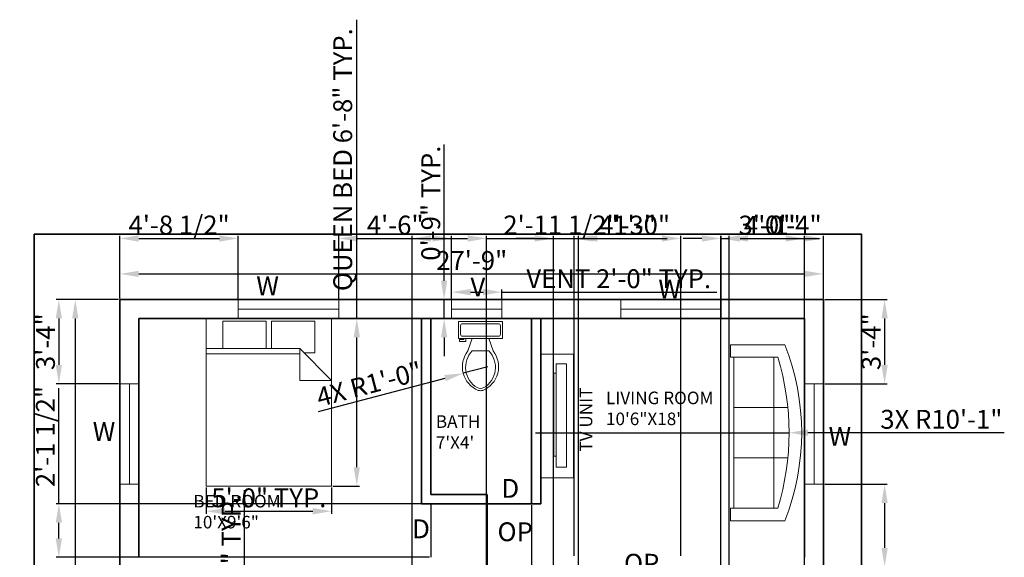
# Model space of a CAD drawing. Units: inches. Extents: x 53076 to 53578, y 41072 to 41816.
# Tile 4 of 4: x 53099 to 53569, y 41560 to 41816. Entities that reach past the tile are written whole.
import ezdxf

# ---------------------------------------------------------------- set-up
doc = ezdxf.new("R2010")
doc.units = ezdxf.units.IN
for name, color, linetype, lineweight in [('A-ANNO-DIMS', 2, 'Continuous', 18), ('A-ANNO-TEXT', 7, 'Continuous', 18), ('A-ANNO-TTLB', 7, 'Continuous', 35), ('A-AREA-IDEN', 7, 'Continuous', 18), ('A-DOOR', 3, 'Continuous', 25), ('A-EQPM', 8, 'Continuous', 18), ('A-FLOR-CASE', 9, 'Continuous', 18), ('A-FLOR-FIXT', 9, 'Continuous', 18), ('A-FURN', 8, 'Continuous', 18), ('A-GLAZ', 4, 'Continuous', 18), ('A-WALL', 7, 'Continuous', 35)]:
    doc.layers.add(name, color=color, linetype=linetype, lineweight=lineweight)
doc.styles.get("Standard").update_dxf_attribs({"font": 'arial.ttf'})
doc.dimstyles.new('ISO-25', dxfattribs={"dimtxt": 9, "dimasz": 9, "dimexe": 1.25, "dimexo": 0.625, "dimtad": 1, "dimdec": 1, "dimrnd": 9, "dimlunit": 3, "dimtxsty": 'Standard', "dimcen": 2.5, "dimadec": 0, "dimazin": 0, "dimtfac": 1, "dimtdec": 1, "dimtmove": 0, "dimatfit": 3, "dimfxl": 1, "dimarcsym": 0})

# ---------------------------------------------------------------- blocks, each defined once
blk = doc.blocks.new('*D1')
at = {"layer": 'A-ANNO-DIMS', "color": 0, "lineweight": -2, "transparency": 16777216}
for p, q in [((53146.81, 41683.28), (53146.81, 41696.2)), ((53482.81, 41683.28), (53482.81, 41696.2)), ((53155.81, 41694.95), (53473.81, 41694.95))]:
    blk.add_line(p, q, dxfattribs=at)
at = {"layer": 'A-ANNO-DIMS', "color": 0, "transparency": 16777216}
for points in [[(53155.81, 41696.45), (53155.81, 41693.45), (53146.81, 41694.95)], [(53473.81, 41696.45), (53473.81, 41693.45), (53482.81, 41694.95)]]:
    blk.add_solid(points, dxfattribs=at)
at = {"layer": 'Defpoints', "color": 0, "transparency": 16777216}
for p in [(53482.81, 41694.95), (53146.81, 41682.66), (53482.81, 41682.66)]:
    blk.add_point(p, dxfattribs=at)
at = {"layer": 'A-ANNO-DIMS', "color": 0, "transparency": 16777216, "insert": (53314.81, 41700.17), "char_height": 9, "attachment_point": 5}
blk.add_mtext('27\'-9"', dxfattribs=at)
blk = doc.blocks.new('*D2')
at = {"layer": 'A-ANNO-DIMS', "color": 0, "lineweight": -2, "transparency": 16777216}
for p, q in [((53146.18, 41682.66), (53124.21, 41682.66)), ((53125.46, 41673.66), (53125.46, 41161.66)), ((53146.18, 41152.66), (53124.21, 41152.66))]:
    blk.add_line(p, q, dxfattribs=at)
at = {"layer": 'A-ANNO-DIMS', "color": 0, "transparency": 16777216}
for points in [[(53123.96, 41673.66), (53126.96, 41673.66), (53125.46, 41682.66)], [(53123.96, 41161.66), (53126.96, 41161.66), (53125.46, 41152.66)]]:
    blk.add_solid(points, dxfattribs=at)
at = {"layer": 'Defpoints', "color": 0, "transparency": 16777216}
for p in [(53146.81, 41682.66), (53125.46, 41152.66), (53146.81, 41152.66)]:
    blk.add_point(p, dxfattribs=at)
at = {"layer": 'A-ANNO-DIMS', "color": 0, "transparency": 16777216, "insert": (53120.23, 41417.66), "char_height": 9, "attachment_point": 5, "rotation": 90}
blk.add_mtext('44\'-3"', dxfattribs=at)
blk = doc.blocks.new('Bed - Queen')
for p, q in [((0, -80.00003), (0, 0)), ((0, 0), (59.99999, 0)), ((59.99999, 0), (59.99999, -80.00003)), ((7.99999, -1.2), (28.79998, -1.2)), ((7.99999, -14.4), (7.99999, -1.2)), ((28.79998, -1.2), (28.79998, -14.4)), ((31.19999, -1.2), (51.99999, -1.2)), ((31.19999, -14.4), (31.19999, -1.2)), ((51.99999, -1.2), (51.99999, -16.4)), ((0, -14.4), (44.8, -14.4)), ((44.8, -16.8), (0, -16.8)), ((59.99999, -29.6), (44.8, -14.4)), ((44.8, -14.4), (44.8, -29.6)), ((51.99999, -16.4), (46.79936, -16.4)), ((44.8, -29.6), (59.99999, -29.6)), ((59.99999, -80.00003), (0, -80.00003))]:
    blk.add_line(p, q)
blk = doc.blocks.new('Sofa - Roundback 7 ft.')
for p, q in [((-12.00002, -32.4421), (-12.00003, -6.5971)), ((11.99997, -32.4421), (11.99998, -6.5971)), ((-36.000027, -34), (-36.000027, -11.4696)), ((-35.999844, -13.3819), (35.9998, -13.3819)), ((35.99998, -34), (35.99998, -11.4696)), ((-36.000027, -32.4421), (35.99998, -32.4421))]:
    blk.add_line(p, q)
for points in [[(-36.000027, -34), (-42.000027, -34), (-42.000027, -8)], [(41.99998, -8), (41.99998, -34), (35.99998, -34)]]:
    blk.add_lwpolyline(points)
for centre, radius, start, end in [((0, -114.25), 114.25, 68.43141, 111.5686), ((-0.00001, -127.1968), 121.1968, 72.72033, 107.2797)]:
    blk.add_arc(centre, radius, start, end)
blk = doc.blocks.new('Toilet - top')
for p, q in [((9.5, -6), (9.5, -2)), ((-10, -8.5), (-8, -8.5)), ((-10, -9.5), (-10, -8.5)), ((-8, -8.5), (-8, -8)), ((-7, -8), (-7, -9.5)), ((-4, -8), (-6, -14)), ((4, -8), (6, -14)), ((-7, -9.5), (-10, -9.5)), ((4, -14), (-4, -14))]:
    blk.add_line(p, q)
blk.add_lwpolyline([(10.5, -8), (10.5, 0), (-10.5, 0), (-10.5, -8)], close=True)
for points in [[(-9.5, -2), (-9.5, -6)], [(8.5, -1), (-8.5, -1)], [(-8.5, -7), (8.5, -7)]]:
    blk.add_lwpolyline(points)
for centre, radius, start, end in [((-8.62, -1.88), 0.884, 81.8699, 188.1301), ((8.62, -1.88), 0.884, 351.8699, 98.1301), ((-8.62, -6.12), 0.884, 171.8699, 278.1301), ((8.62, -6.12), 0.884, 261.8699, 8.1301), ((3.52, -21.58), 12.17, 141.4691, 247.9714), ((4.2, -21.82), 11.33, 136.3677, 238.9468), ((-3.52, -21.58), 12.17, 292.0284, 38.5307), ((-4.2, -21.82), 11.33, 301.053, 43.6321), ((0, -27.88), 4, 245.7318, 294.2682), ((0, -29), 4, 254.8605, 285.1395)]:
    blk.add_arc(centre, radius, start, end)
blk = doc.blocks.new('WIN-48IN')
for p, q in [((0, 48), (9, 48)), ((4.5, 48), (4.5, 0)), ((0, 0), (9, 0))]:
    blk.add_line(p, q)
blk = doc.blocks.new('VENT-24IN')
for p, q in [((0, 9), (0, 0)), ((24, 9), (24, 0)), ((0, 4.5), (24, 4.5))]:
    blk.add_line(p, q)
blk = doc.blocks.new('*D18')
at = {"layer": 'A-ANNO-DIMS', "color": 0, "lineweight": -2, "transparency": 16777216}
for p, q in [((53206.33, 41493.74), (53206.33, 41591.64)), ((53207.95, 41484.74), (53205.08, 41484.74)), ((53206.33, 41469.74), (53206.33, 41484.74)), ((53207.95, 41469.74), (53205.08, 41469.74)), ((53206.33, 41460.74), (53206.33, 41451.74))]:
    blk.add_line(p, q, dxfattribs=at)
at = {"layer": 'A-ANNO-DIMS', "color": 0, "transparency": 16777216}
for points in [[(53204.83, 41493.74), (53207.83, 41493.74), (53206.33, 41484.74)], [(53204.83, 41460.74), (53207.83, 41460.74), (53206.33, 41469.74)]]:
    blk.add_solid(points, dxfattribs=at)
at = {"layer": 'Defpoints', "color": 0, "transparency": 16777216}
for p in [(53206.33, 41484.74), (53208.58, 41484.74), (53208.58, 41469.74)]:
    blk.add_point(p, dxfattribs=at)
at = {"layer": 'A-ANNO-DIMS', "color": 0, "transparency": 16777216, "insert": (53201.05, 41547.19), "char_height": 9, "attachment_point": 5, "rotation": 90}
blk.add_mtext('SINK 1\'-3" TYP.', dxfattribs=at)
blk = doc.blocks.new('*D24')
at = {"layer": 'A-ANNO-DIMS', "color": 0, "lineweight": -2, "transparency": 16777216}
for p, q in [((53305.23, 41683.28), (53305.23, 41687.51)), ((53314.23, 41686.26), (53320.23, 41686.26)), ((53329.23, 41683.28), (53329.23, 41687.51)), ((53329.23, 41686.26), (53431.83, 41686.26))]:
    blk.add_line(p, q, dxfattribs=at)
at = {"layer": 'A-ANNO-DIMS', "color": 0, "transparency": 16777216}
for points in [[(53314.23, 41687.76), (53314.23, 41684.76), (53305.23, 41686.26)], [(53320.23, 41687.76), (53320.23, 41684.76), (53329.23, 41686.26)]]:
    blk.add_solid(points, dxfattribs=at)
at = {"layer": 'Defpoints', "color": 0, "transparency": 16777216}
for p in [(53329.23, 41686.26), (53305.23, 41682.66), (53329.23, 41682.66)]:
    blk.add_point(p, dxfattribs=at)
at = {"layer": 'A-ANNO-DIMS', "color": 0, "transparency": 16777216, "insert": (53385.03, 41691.48), "char_height": 9, "attachment_point": 5}
blk.add_mtext('VENT 2\'-0" TYP.', dxfattribs=at)
blk = doc.blocks.new('*D25')
at = {"layer": 'A-ANNO-DIMS', "color": 0, "lineweight": -2, "transparency": 16777216}
for p, q in [((53301.63, 41691.66), (53301.63, 41756.77)), ((53304.61, 41682.66), (53300.38, 41682.66)), ((53301.63, 41673.66), (53301.63, 41682.66)), ((53304.61, 41673.66), (53300.38, 41673.66)), ((53301.63, 41664.66), (53301.63, 41655.66))]:
    blk.add_line(p, q, dxfattribs=at)
at = {"layer": 'A-ANNO-DIMS', "color": 0, "transparency": 16777216}
for points in [[(53300.13, 41691.66), (53303.13, 41691.66), (53301.63, 41682.66)], [(53300.13, 41664.66), (53303.13, 41664.66), (53301.63, 41673.66)]]:
    blk.add_solid(points, dxfattribs=at)
at = {"layer": 'Defpoints', "color": 0, "transparency": 16777216}
for p in [(53301.63, 41682.66), (53305.23, 41682.66), (53305.23, 41673.66)]:
    blk.add_point(p, dxfattribs=at)
at = {"layer": 'A-ANNO-DIMS', "color": 0, "transparency": 16777216, "insert": (53296.41, 41728.71), "char_height": 9, "attachment_point": 5, "rotation": 90}
blk.add_mtext('0\'-9" TYP.', dxfattribs=at)
blk = doc.blocks.new('*D26')
at = {"layer": 'A-ANNO-DIMS', "color": 0, "lineweight": -2, "transparency": 16777216}
for p, q in [((53259.91, 41673.66), (53259.91, 41816.3)), ((53248.53, 41673.66), (53261.16, 41673.66)), ((53259.91, 41602.66), (53259.91, 41664.66)), ((53248.53, 41593.66), (53261.16, 41593.66))]:
    blk.add_line(p, q, dxfattribs=at)
at = {"layer": 'A-ANNO-DIMS', "color": 0, "transparency": 16777216}
for points in [[(53258.41, 41664.66), (53261.41, 41664.66), (53259.91, 41673.66)], [(53258.41, 41602.66), (53261.41, 41602.66), (53259.91, 41593.66)]]:
    blk.add_solid(points, dxfattribs=at)
at = {"layer": 'Defpoints', "color": 0, "transparency": 16777216}
for p in [(53247.91, 41673.66), (53259.91, 41673.66), (53247.91, 41593.66)]:
    blk.add_point(p, dxfattribs=at)
at = {"layer": 'A-ANNO-DIMS', "color": 0, "transparency": 16777216, "insert": (53254.35, 41749.48), "char_height": 9, "attachment_point": 5, "rotation": 90}
blk.add_mtext('QUEEN BED 6\'-8" TYP.', dxfattribs=at)
blk = doc.blocks.new('*D27')
at = {"layer": 'A-ANNO-DIMS', "color": 0, "lineweight": -2, "transparency": 16777216}
for p, q in [((53187.91, 41593.03), (53187.91, 41580.41)), ((53247.91, 41593.03), (53247.91, 41580.41)), ((53196.91, 41581.66), (53238.91, 41581.66))]:
    blk.add_line(p, q, dxfattribs=at)
at = {"layer": 'A-ANNO-DIMS', "color": 0, "transparency": 16777216}
for points in [[(53196.91, 41583.16), (53196.91, 41580.16), (53187.91, 41581.66)], [(53238.91, 41583.16), (53238.91, 41580.16), (53247.91, 41581.66)]]:
    blk.add_solid(points, dxfattribs=at)
at = {"layer": 'Defpoints', "color": 0, "transparency": 16777216}
for p in [(53187.91, 41593.66), (53247.91, 41593.66), (53247.91, 41581.66)]:
    blk.add_point(p, dxfattribs=at)
at = {"layer": 'A-ANNO-DIMS', "color": 0, "transparency": 16777216, "insert": (53217.91, 41586.88), "char_height": 9, "attachment_point": 5}
blk.add_mtext('5\'-0" TYP.', dxfattribs=at)
blk = doc.blocks.new('*D32')
at = {"layer": 'A-ANNO-DIMS', "color": 0, "lineweight": -2, "transparency": 16777216}
for p, q in [((53483.43, 41594.51), (53513.26, 41594.51)), ((53512.01, 41585.51), (53512.01, 41564.16)), ((53483.43, 41555.16), (53513.26, 41555.16)), ((53512.01, 41555.16), (53512.01, 41500.02))]:
    blk.add_line(p, q, dxfattribs=at)
at = {"layer": 'A-ANNO-DIMS', "color": 0, "transparency": 16777216}
for points in [[(53510.51, 41585.51), (53513.51, 41585.51), (53512.01, 41594.51)], [(53510.51, 41564.16), (53513.51, 41564.16), (53512.01, 41555.16)]]:
    blk.add_solid(points, dxfattribs=at)
at = {"layer": 'Defpoints', "color": 0, "transparency": 16777216}
for p in [(53482.81, 41594.51), (53482.81, 41555.16), (53512.01, 41555.16)]:
    blk.add_point(p, dxfattribs=at)
at = {"layer": 'A-ANNO-DIMS', "color": 0, "transparency": 16777216, "insert": (53506.72, 41523.09), "char_height": 9, "attachment_point": 5, "rotation": 90}
blk.add_mtext('3\'-3 1/2"', dxfattribs=at)
blk = doc.blocks.new('*D39')
at = {"layer": 'A-ANNO-DIMS', "color": 0, "lineweight": -2, "transparency": 16777216}
for p, q in [((53146.81, 41683.28), (53146.81, 41713.11)), ((53155.81, 41711.86), (53194.3, 41711.86)), ((53203.3, 41683.28), (53203.3, 41713.11))]:
    blk.add_line(p, q, dxfattribs=at)
at = {"layer": 'A-ANNO-DIMS', "color": 0, "transparency": 16777216}
for points in [[(53155.81, 41713.36), (53155.81, 41710.36), (53146.81, 41711.86)], [(53194.3, 41713.36), (53194.3, 41710.36), (53203.3, 41711.86)]]:
    blk.add_solid(points, dxfattribs=at)
at = {"layer": 'Defpoints', "color": 0, "transparency": 16777216}
for p in [(53203.3, 41711.86), (53146.81, 41682.66), (53203.3, 41682.66)]:
    blk.add_point(p, dxfattribs=at)
at = {"layer": 'A-ANNO-DIMS', "color": 0, "transparency": 16777216, "insert": (53175.05, 41717.13), "char_height": 9, "attachment_point": 5}
blk.add_mtext('4\'-8 1/2"', dxfattribs=at)
blk = doc.blocks.new('*D40')
at = {"layer": 'A-ANNO-DIMS', "color": 0, "lineweight": -2, "transparency": 16777216}
for p, q in [((53251.3, 41683.28), (53251.3, 41713.11)), ((53260.3, 41711.86), (53296.23, 41711.86)), ((53305.23, 41683.28), (53305.23, 41713.11))]:
    blk.add_line(p, q, dxfattribs=at)
at = {"layer": 'A-ANNO-DIMS', "color": 0, "transparency": 16777216}
for points in [[(53260.3, 41713.36), (53260.3, 41710.36), (53251.3, 41711.86)], [(53296.23, 41713.36), (53296.23, 41710.36), (53305.23, 41711.86)]]:
    blk.add_solid(points, dxfattribs=at)
at = {"layer": 'Defpoints', "color": 0, "transparency": 16777216}
for p in [(53305.23, 41711.86), (53251.3, 41682.66), (53305.23, 41682.66)]:
    blk.add_point(p, dxfattribs=at)
at = {"layer": 'A-ANNO-DIMS', "color": 0, "transparency": 16777216, "insert": (53278.27, 41717.08), "char_height": 9, "attachment_point": 5}
blk.add_mtext('4\'-6"', dxfattribs=at)
blk = doc.blocks.new('*D41')
at = {"layer": 'A-ANNO-DIMS', "color": 0, "lineweight": -2, "transparency": 16777216}
for p, q in [((53433.98, 41683.28), (53433.98, 41713.11)), ((53442.98, 41711.86), (53473.81, 41711.86)), ((53482.81, 41683.28), (53482.81, 41713.11))]:
    blk.add_line(p, q, dxfattribs=at)
at = {"layer": 'A-ANNO-DIMS', "color": 0, "transparency": 16777216}
for points in [[(53442.98, 41713.36), (53442.98, 41710.36), (53433.98, 41711.86)], [(53473.81, 41713.36), (53473.81, 41710.36), (53482.81, 41711.86)]]:
    blk.add_solid(points, dxfattribs=at)
at = {"layer": 'Defpoints', "color": 0, "transparency": 16777216}
for p in [(53482.81, 41711.86), (53433.98, 41682.66), (53482.81, 41682.66)]:
    blk.add_point(p, dxfattribs=at)
at = {"layer": 'A-ANNO-DIMS', "color": 0, "transparency": 16777216, "insert": (53458.4, 41717), "char_height": 9, "attachment_point": 5}
blk.add_mtext('4\'-1"', dxfattribs=at)
blk = doc.blocks.new('*D45')
at = {"layer": 'A-ANNO-DIMS', "color": 0, "lineweight": -2, "transparency": 16777216}
for p, q in [((53146.18, 41682.66), (53116.36, 41682.66)), ((53117.61, 41673.66), (53117.61, 41651.51)), ((53146.18, 41642.51), (53116.36, 41642.51))]:
    blk.add_line(p, q, dxfattribs=at)
at = {"layer": 'A-ANNO-DIMS', "color": 0, "transparency": 16777216}
for points in [[(53116.11, 41673.66), (53119.11, 41673.66), (53117.61, 41682.66)], [(53116.11, 41651.51), (53119.11, 41651.51), (53117.61, 41642.51)]]:
    blk.add_solid(points, dxfattribs=at)
at = {"layer": 'Defpoints', "color": 0, "transparency": 16777216}
for p in [(53146.81, 41682.66), (53117.61, 41642.51), (53146.81, 41642.51)]:
    blk.add_point(p, dxfattribs=at)
at = {"layer": 'A-ANNO-DIMS', "color": 0, "transparency": 16777216, "insert": (53112.38, 41662.58), "char_height": 9, "attachment_point": 5, "rotation": 90}
blk.add_mtext('3\'-4"', dxfattribs=at)
blk = doc.blocks.new('*D48')
at = {"layer": 'A-ANNO-DIMS', "color": 0, "lineweight": -2, "transparency": 16777216}
for p, q in [((53483.43, 41682.66), (53513.26, 41682.66)), ((53512.01, 41673.66), (53512.01, 41651.51)), ((53483.43, 41642.51), (53513.26, 41642.51))]:
    blk.add_line(p, q, dxfattribs=at)
at = {"layer": 'A-ANNO-DIMS', "color": 0, "transparency": 16777216}
for points in [[(53510.51, 41673.66), (53513.51, 41673.66), (53512.01, 41682.66)], [(53510.51, 41651.51), (53513.51, 41651.51), (53512.01, 41642.51)]]:
    blk.add_solid(points, dxfattribs=at)
at = {"layer": 'Defpoints', "color": 0, "transparency": 16777216}
for p in [(53482.81, 41682.66), (53482.81, 41642.51), (53512.01, 41642.51)]:
    blk.add_point(p, dxfattribs=at)
at = {"layer": 'A-ANNO-DIMS', "color": 0, "transparency": 16777216, "insert": (53506.78, 41662.58), "char_height": 9, "attachment_point": 5, "rotation": 90}
blk.add_mtext('3\'-4"', dxfattribs=at)
blk = doc.blocks.new('*D52')
at = {"layer": 'A-ANNO-DIMS', "color": 0, "lineweight": -2, "transparency": 16777216}
for p, q in [((53363.81, 41560.28), (53363.81, 41713.11)), ((53372.81, 41711.86), (53405.67, 41711.86)), ((53414.67, 41560.28), (53414.67, 41713.11))]:
    blk.add_line(p, q, dxfattribs=at)
at = {"layer": 'A-ANNO-DIMS', "color": 0, "transparency": 16777216}
for points in [[(53372.81, 41713.36), (53372.81, 41710.36), (53363.81, 41711.86)], [(53405.67, 41713.36), (53405.67, 41710.36), (53414.67, 41711.86)]]:
    blk.add_solid(points, dxfattribs=at)
at = {"layer": 'Defpoints', "color": 0, "transparency": 16777216}
for p in [(53414.67, 41711.86), (53363.81, 41559.66), (53414.67, 41559.66)]:
    blk.add_point(p, dxfattribs=at)
at = {"layer": 'A-ANNO-DIMS', "color": 0, "transparency": 16777216, "insert": (53389.24, 41717.08), "char_height": 9, "attachment_point": 5}
blk.add_mtext('4\'-3"', dxfattribs=at)
blk = doc.blocks.new('*D55')
at = {"layer": 'A-ANNO-DIMS', "color": 0, "lineweight": -2, "transparency": 16777216}
for p, q in [((53322.2, 41589.03), (53322.2, 41122.21)), ((53343.31, 41584.53), (53343.31, 41122.21)), ((53331.2, 41123.46), (53334.31, 41123.46)), ((53343.31, 41123.46), (53376.63, 41123.46))]:
    blk.add_line(p, q, dxfattribs=at)
at = {"layer": 'A-ANNO-DIMS', "color": 0, "transparency": 16777216}
for points in [[(53331.2, 41124.96), (53331.2, 41121.96), (53322.2, 41123.46)], [(53334.31, 41124.96), (53334.31, 41121.96), (53343.31, 41123.46)]]:
    blk.add_solid(points, dxfattribs=at)
at = {"layer": 'Defpoints', "color": 0, "transparency": 16777216}
for p in [(53322.2, 41589.66), (53343.31, 41585.16), (53343.31, 41123.46)]:
    blk.add_point(p, dxfattribs=at)
at = {"layer": 'A-ANNO-DIMS', "color": 0, "transparency": 16777216, "insert": (53364.47, 41128.68), "char_height": 9, "attachment_point": 5}
blk.add_mtext('1\'-9"', dxfattribs=at)
blk = doc.blocks.new('*D56')
at = {"layer": 'A-ANNO-DIMS', "color": 0, "lineweight": -2, "transparency": 16777216}
for p, q in [((53117.61, 41585.16), (53117.61, 41640.46)), ((53294.68, 41585.16), (53116.36, 41585.16)), ((53117.61, 41568.66), (53117.61, 41576.16)), ((53294.68, 41559.66), (53116.36, 41559.66))]:
    blk.add_line(p, q, dxfattribs=at)
at = {"layer": 'A-ANNO-DIMS', "color": 0, "transparency": 16777216}
for points in [[(53116.11, 41576.16), (53119.11, 41576.16), (53117.61, 41585.16)], [(53116.11, 41568.66), (53119.11, 41568.66), (53117.61, 41559.66)]]:
    blk.add_solid(points, dxfattribs=at)
at = {"layer": 'Defpoints', "color": 0, "transparency": 16777216}
for p in [(53117.61, 41585.16), (53295.31, 41585.16), (53295.31, 41559.66)]:
    blk.add_point(p, dxfattribs=at)
at = {"layer": 'A-ANNO-DIMS', "color": 0, "transparency": 16777216, "insert": (53112.33, 41617.31), "char_height": 9, "attachment_point": 5, "rotation": 90}
blk.add_mtext('2\'-1 1/2"', dxfattribs=at)
blk = doc.blocks.new('*D60')
at = {"layer": 'A-ANNO-DIMS', "color": 0, "lineweight": -2, "transparency": 16777216}
for p, q in [((53286.43, 41391.78), (53286.43, 41713.11)), ((53295.43, 41711.86), (53312.81, 41711.86)), ((53321.81, 41374.01), (53321.81, 41713.11)), ((53321.81, 41711.86), (53384.1, 41711.86))]:
    blk.add_line(p, q, dxfattribs=at)
at = {"layer": 'A-ANNO-DIMS', "color": 0, "transparency": 16777216}
for points in [[(53295.43, 41713.36), (53295.43, 41710.36), (53286.43, 41711.86)], [(53312.81, 41713.36), (53312.81, 41710.36), (53321.81, 41711.86)]]:
    blk.add_solid(points, dxfattribs=at)
at = {"layer": 'Defpoints', "color": 0, "transparency": 16777216}
for p in [(53321.81, 41711.86), (53286.43, 41391.16), (53321.81, 41373.39)]:
    blk.add_point(p, dxfattribs=at)
at = {"layer": 'A-ANNO-DIMS', "color": 0, "transparency": 16777216, "insert": (53357.45, 41717.13), "char_height": 9, "attachment_point": 5}
blk.add_mtext('2\'-11 1/2"', dxfattribs=at)
blk = doc.blocks.new('*D61')
at = {"layer": 'A-ANNO-DIMS', "color": 0, "lineweight": -2, "transparency": 16777216}
for p, q in [((53437.81, 41380.28), (53437.81, 41713.11)), ((53446.81, 41711.86), (53464.81, 41711.86)), ((53473.81, 41380.28), (53473.81, 41713.11))]:
    blk.add_line(p, q, dxfattribs=at)
at = {"layer": 'A-ANNO-DIMS', "color": 0, "transparency": 16777216}
for points in [[(53446.81, 41713.36), (53446.81, 41710.36), (53437.81, 41711.86)], [(53464.81, 41713.36), (53464.81, 41710.36), (53473.81, 41711.86)]]:
    blk.add_solid(points, dxfattribs=at)
at = {"layer": 'Defpoints', "color": 0, "transparency": 16777216}
for p in [(53473.81, 41711.86), (53437.81, 41379.66), (53473.81, 41379.66)]:
    blk.add_point(p, dxfattribs=at)
at = {"layer": 'A-ANNO-DIMS', "color": 0, "transparency": 16777216, "insert": (53455.81, 41717.08), "char_height": 9, "attachment_point": 5}
blk.add_mtext('3\'-0"', dxfattribs=at)
blk = doc.blocks.new('*D62')
at = {"layer": 'A-ANNO-DIMS', "color": 0, "lineweight": -2, "transparency": 16777216}
for p, q in [((53344.81, 41711.86), (53335.81, 41711.86)), ((53353.81, 41448.78), (53353.81, 41713.11)), ((53353.81, 41711.86), (53365.81, 41711.86)), ((53365.81, 41448.78), (53365.81, 41713.11)), ((53374.81, 41711.86), (53408.13, 41711.86))]:
    blk.add_line(p, q, dxfattribs=at)
at = {"layer": 'A-ANNO-DIMS', "color": 0, "transparency": 16777216}
for points in [[(53344.81, 41713.36), (53344.81, 41710.36), (53353.81, 41711.86)], [(53374.81, 41713.36), (53374.81, 41710.36), (53365.81, 41711.86)]]:
    blk.add_solid(points, dxfattribs=at)
at = {"layer": 'Defpoints', "color": 0, "transparency": 16777216}
for p in [(53365.81, 41711.86), (53353.81, 41448.16), (53365.81, 41448.16)]:
    blk.add_point(p, dxfattribs=at)
at = {"layer": 'A-ANNO-DIMS', "color": 0, "transparency": 16777216, "insert": (53395.97, 41717.08), "char_height": 9, "attachment_point": 5}
blk.add_mtext('1\'-0"', dxfattribs=at)
blk = doc.blocks.new('*D67')
at = {"layer": 'A-ANNO-DIMS', "color": 0, "lineweight": -2, "transparency": 16777216}
for p, q in [((53424.78, 41711.86), (53415.78, 41711.86)), ((53433.78, 41514.52), (53433.78, 41713.11)), ((53433.78, 41711.86), (53437.81, 41711.86)), ((53437.81, 41517.49), (53437.81, 41713.11)), ((53446.81, 41711.86), (53480.98, 41711.86))]:
    blk.add_line(p, q, dxfattribs=at)
at = {"layer": 'A-ANNO-DIMS', "color": 0, "transparency": 16777216}
for points in [[(53424.78, 41713.36), (53424.78, 41710.36), (53433.78, 41711.86)], [(53446.81, 41713.36), (53446.81, 41710.36), (53437.81, 41711.86)]]:
    blk.add_solid(points, dxfattribs=at)
at = {"layer": 'Defpoints', "color": 0, "transparency": 16777216}
for p in [(53437.81, 41711.86), (53437.81, 41516.86), (53433.78, 41513.89)]:
    blk.add_point(p, dxfattribs=at)
at = {"layer": 'A-ANNO-DIMS', "color": 0, "transparency": 16777216, "insert": (53468.39, 41717.08), "char_height": 9, "attachment_point": 5}
blk.add_mtext('0\'-4"', dxfattribs=at)
blk = doc.blocks.new('*D71')
at = {"layer": 'A-ANNO-DIMS', "color": 0, "lineweight": -2, "transparency": 16777216}
for p, q in [((53345.22, 41619.13), (53466.41, 41619.13)), ((53569.19, 41619.13), (53475.41, 41619.13))]:
    blk.add_line(p, q, dxfattribs=at)
at = {"layer": 'A-ANNO-DIMS', "color": 0, "transparency": 16777216}
blk.add_solid([(53475.41, 41620.63), (53475.41, 41617.63), (53466.41, 41619.13)], dxfattribs=at)
at = {"layer": 'Defpoints', "color": 0, "transparency": 16777216}
for p in [(53345.22, 41619.13), (53466.41, 41619.13)]:
    blk.add_point(p, dxfattribs=at)
at = {"layer": 'A-ANNO-DIMS', "color": 0, "transparency": 16777216, "insert": (53539.13, 41624.36), "char_height": 9, "attachment_point": 5, "rotation": 0.0001}
blk.add_mtext('3X R10\'-1"', dxfattribs=at)
blk = doc.blocks.new('*D73')
at = {"layer": 'A-ANNO-DIMS', "color": 0, "lineweight": -2, "transparency": 16777216}
for p, q in [((53322.53, 41650.59), (53310.76, 41647.5)), ((53241.62, 41629.33), (53302.05, 41645.21))]:
    blk.add_line(p, q, dxfattribs=at)
at = {"layer": 'A-ANNO-DIMS', "color": 0, "transparency": 16777216}
blk.add_solid([(53301.67, 41646.66), (53302.44, 41643.76), (53310.76, 41647.5)], dxfattribs=at)
at = {"layer": 'Defpoints', "color": 0, "transparency": 16777216}
for p in [(53322.53, 41650.59), (53310.76, 41647.5)]:
    blk.add_point(p, dxfattribs=at)
at = {"layer": 'A-ANNO-DIMS', "color": 0, "transparency": 16777216, "insert": (53266.16, 41641.18), "char_height": 9, "attachment_point": 5, "rotation": 14.7186}
blk.add_mtext('4X R1\'-0"', dxfattribs=at)

msp = doc.modelspace()

# ---------------------------------------------------------------- linework, layer by layer
at = {"layer": 'A-ANNO-TTLB'}
msp.add_lwpolyline([(53105.85, 41713.9), (53500.98, 41713.9), (53500.98, 41125.46), (53105.85, 41125.46)], close=True, dxfattribs=at)
at = {"layer": 'A-DOOR'}
msp.add_line((53295.31, 41585.16), (53295.31, 41559.66), dxfattribs=at)
at = {"layer": 'A-EQPM'}
for p, q in [((53355.19, 41647.62), (53354.03, 41647.62)), ((53354.03, 41647.62), (53354.03, 41607.91)), ((53354.03, 41607.91), (53355.19, 41607.91))]:
    msp.add_line(p, q, dxfattribs=at)
msp.add_lwpolyline([(53355.19, 41652.09), (53360.11, 41652.09), (53360.11, 41602.64), (53355.19, 41602.64)], close=True, dxfattribs=at)
at = {"layer": 'A-FLOR-CASE'}
for p, q in [((53347.81, 41656.62), (53347.81, 41656.62)), ((53347.81, 41656.62), (53363.41, 41656.62)), ((53363.41, 41656.62), (53363.41, 41597.58)), ((53363.41, 41597.58), (53347.81, 41597.58))]:
    msp.add_line(p, q, dxfattribs=at)
at = {"layer": 'A-WALL'}
for p, q in [((53146.81, 41152.66), (53146.81, 41682.66)), ((53146.81, 41682.66), (53482.81, 41682.66)), ((53482.81, 41682.66), (53482.81, 41370.66)), ((53155.81, 41673.66), (53473.81, 41673.66)), ((53155.81, 41559.66), (53155.81, 41673.66)), ((53290.81, 41673.66), (53290.81, 41585.16)), ((53295.31, 41673.66), (53295.31, 41589.66)), ((53343.31, 41673.66), (53343.31, 41585.16)), ((53347.81, 41673.66), (53347.81, 41585.16)), ((53473.81, 41673.66), (53473.81, 41559.66)), ((53295.31, 41589.66), (53322.2, 41589.66)), ((53322.2, 41589.66), (53322.2, 41585.16)), ((53290.81, 41585.16), (53347.81, 41585.16))]:
    msp.add_line(p, q, dxfattribs=at)

# ---------------------------------------------------------------- block references
at = {"layer": 'A-FLOR-FIXT'}
msp.add_blockref('Toilet - top', (53319.01, 41672.17), dxfattribs=at)
at = {"layer": 'A-FURN'}
msp.add_blockref('Bed - Queen', (53187.91, 41673.66), dxfattribs=at)
at = {"layer": 'A-FURN', "rotation": 270}
msp.add_blockref('Sofa - Roundback 7 ft.', (53472.41, 41619.13), dxfattribs=at)
at = {"layer": 'A-GLAZ', "rotation": 270}
for p in [(53203.3, 41682.66), (53385.98, 41682.66)]:
    msp.add_blockref('WIN-48IN', p, dxfattribs=at)
at = {"layer": 'A-GLAZ'}
for name, p in [('VENT-24IN', (53305.23, 41673.66)), ('WIN-48IN', (53146.81, 41594.5)), ('WIN-48IN', (53473.81, 41594.5))]:
    msp.add_blockref(name, p, dxfattribs=at)

# ---------------------------------------------------------------- texts
at = {"layer": 'A-ANNO-TEXT', "char_height": 9, "attachment_point": 1}
for s, insert in [('W ', (53211.93, 41693.73)), ('V ', (53314.2, 41693.2)), ('W ', (53403.94, 41692.23)), ('W ', (53133.78, 41624.21)), ('W ', (53485.25, 41621.88)), ('D ', (53329.02, 41597.06)), ('D ', (53286.37, 41577.74)), ('OP ', (53327.13, 41576.34)), ('OP ', (53387.55, 41561.31))]:
    msp.add_mtext_dynamic_manual_height_columns(s, width=6.4326, gutter_width=12.5, heights=[0], dxfattribs=dict(at, insert=insert))
at = {"layer": 'A-ANNO-TEXT', "insert": (53366.38, 41610.13), "char_height": 6, "attachment_point": 1, "rotation": 90}
msp.add_mtext_dynamic_manual_height_columns('TV UNIT', width=85.6025, gutter_width=12.5, heights=[0], dxfattribs=at)
at = {"layer": 'A-AREA-IDEN', "char_height": 6, "attachment_point": 1}
for s, insert in [('LIVING ROOM\\P10\'6"X18\'', (53378.94, 41638.75)), ("BATH\\P7'X4'", (53297.67, 41627.46)), ('BED ROOM\\P10\'X9\'6"', (53181.86, 41589.44))]:
    msp.add_mtext_dynamic_manual_height_columns(s, width=85.6025, gutter_width=12.5, heights=[0], dxfattribs=dict(at, insert=insert))

# ---------------------------------------------------------------- dimensions: what is measured, and where the dimension line sits
at = {"layer": 'A-ANNO-DIMS'}
for base, p1, p2, text, picture, middle in [((53259.91, 41673.66), (53247.91, 41593.66), (53247.91, 41673.66), 'QUEEN BED <> TYP.', '*D26', (53254.35, 41749.48)), ((53301.63, 41682.66), (53305.23, 41673.66), (53305.23, 41682.66), '<> TYP.', '*D25', (53296.41, 41728.71)), ((53206.33, 41484.74), (53208.58, 41469.74), (53208.58, 41484.74), 'SINK <> TYP.', '*D18', (53201.05, 41547.19))]:
    dim = msp.add_linear_dim(base=base, p1=p1, p2=p2, angle=90, text=text, dimstyle='ISO-25', override={"dimdec": 1, "dimlfac": 1, "dimrnd": 0, "dimzin": 1, "dimdsep": 46, "dimlunit": 4, "dimfrac": 2}, dxfattribs=at)
    dim.commit()
    dim.dimension.update_dxf_attribs({"geometry": picture, "text_midpoint": middle})
for base, p1, p2, override, picture, middle in [((53203.3, 41711.86), (53146.81, 41682.66), (53203.3, 41682.66), {"dimdec": 1, "dimlfac": 1, "dimrnd": 0, "dimzin": 1, "dimdsep": 46, "dimlunit": 4, "dimfrac": 2}, '*D39', (53175.05, 41717.13)), ((53321.81, 41711.86), (53286.43, 41391.16), (53321.81, 41373.39), {"dimdec": 1, "dimlfac": 1, "dimrnd": 0, "dimzin": 1, "dimdsep": 46, "dimlunit": 4, "dimfrac": 2}, '*D60', (53357.45, 41717.13)), ((53305.23, 41711.86), (53251.3, 41682.66), (53305.23, 41682.66), {"dimdec": 1, "dimlfac": 1, "dimrnd": 0, "dimzin": 1, "dimdsep": 46, "dimlunit": 4, "dimfrac": 2}, '*D40', (53278.27, 41717.08)), ((53365.81, 41711.86), (53353.81, 41448.16), (53365.81, 41448.16), {"dimdec": 1, "dimlfac": 1, "dimrnd": 0, "dimzin": 1, "dimdsep": 46, "dimlunit": 4, "dimfrac": 2}, '*D62', (53395.97, 41717.08)), ((53414.67, 41711.86), (53363.81, 41559.66), (53414.67, 41559.66), {"dimdec": 1, "dimlfac": 1, "dimrnd": 0, "dimzin": 1, "dimdsep": 46, "dimlunit": 4, "dimfrac": 2}, '*D52', (53389.24, 41717.08)), ((53437.81, 41711.86), (53433.78, 41513.89), (53437.81, 41516.86), {"dimdec": 1, "dimlfac": 1, "dimrnd": 0, "dimzin": 1, "dimdsep": 46, "dimlunit": 4, "dimfrac": 2}, '*D67', (53468.39, 41717.08)), ((53482.81, 41711.86), (53433.98, 41682.66), (53482.81, 41682.66), {"dimdec": 1, "dimlfac": 1, "dimrnd": 0, "dimzin": 1, "dimdsep": 46, "dimlunit": 4, "dimfrac": 2}, '*D41', (53458.4, 41717)), ((53473.81, 41711.86), (53437.81, 41379.66), (53473.81, 41379.66), {"dimdec": 1, "dimlfac": 1, "dimrnd": 0, "dimzin": 1, "dimdsep": 46, "dimlunit": 4, "dimfrac": 2}, '*D61', (53455.81, 41717.08)), ((53482.81, 41694.95), (53146.81, 41682.66), (53482.81, 41682.66), {"dimclrd": 0, "dimclre": 0, "dimclrt": 0}, '*D1', (53314.81, 41700.17)), ((53343.31, 41123.46), (53322.2, 41589.66), (53343.31, 41585.16), {"dimdec": 1, "dimlfac": 1, "dimrnd": 0, "dimzin": 1, "dimdsep": 46, "dimlunit": 4, "dimfrac": 2}, '*D55', (53364.47, 41128.68))]:
    dim = msp.add_linear_dim(base=base, p1=p1, p2=p2, dimstyle='ISO-25', override=override, dxfattribs=at)
    dim.commit()
    dim.dimension.update_dxf_attribs({"geometry": picture, "text_midpoint": middle})
for base, p1, p2, text, picture, middle in [((53329.23, 41686.26), (53305.23, 41682.66), (53329.23, 41682.66), 'VENT <> TYP.', '*D24', (53385.03, 41691.48)), ((53247.91, 41581.66), (53187.91, 41593.66), (53247.91, 41593.66), '<> TYP.', '*D27', (53217.91, 41586.88))]:
    dim = msp.add_linear_dim(base=base, p1=p1, p2=p2, text=text, dimstyle='ISO-25', override={"dimdec": 1, "dimlfac": 1, "dimrnd": 0, "dimzin": 1, "dimdsep": 46, "dimlunit": 4, "dimfrac": 2}, dxfattribs=at)
    dim.commit()
    dim.dimension.update_dxf_attribs({"geometry": picture, "text_midpoint": middle})
for base, p1, p2, override, picture, middle in [((53117.6064, 41642.5051), (53146.8064, 41682.656), (53146.8064, 41642.5051), {"dimdec": 1, "dimlfac": 1, "dimrnd": 0, "dimzin": 1, "dimdsep": 46, "dimlunit": 4, "dimfrac": 2}, '*D45', (53112.3832, 41662.5806)), ((53125.46, 41152.66), (53146.81, 41682.66), (53146.81, 41152.66), {"dimclrd": 0, "dimclre": 0, "dimclrt": 0}, '*D2', (53120.23, 41417.66)), ((53512.0064, 41642.5051), (53482.8064, 41682.656), (53482.8064, 41642.5051), {"dimdec": 1, "dimlfac": 1, "dimrnd": 0, "dimzin": 1, "dimdsep": 46, "dimlunit": 4, "dimfrac": 2}, '*D48', (53506.7832, 41662.5806)), ((53117.61, 41585.16), (53295.31, 41559.66), (53295.31, 41585.16), {"dimdec": 1, "dimlfac": 1, "dimrnd": 0, "dimzin": 1, "dimdsep": 46, "dimlunit": 4, "dimfrac": 2}, '*D56', (53112.33, 41617.31)), ((53512.0064, 41555.156), (53482.8064, 41594.5051), (53482.8064, 41555.156), {"dimdec": 1, "dimlfac": 1, "dimrnd": 0, "dimzin": 1, "dimdsep": 46, "dimlunit": 4, "dimfrac": 2}, '*D32', (53506.7248, 41523.0863))]:
    dim = msp.add_linear_dim(base=base, p1=p1, p2=p2, angle=90, dimstyle='ISO-25', override=override, dxfattribs=at)
    dim.commit()
    dim.dimension.update_dxf_attribs({"geometry": picture, "text_midpoint": middle})
dim = msp.add_radius_dim(center=(53322.53, 41650.59), mpoint=(53310.76, 41647.5), text='4X <>', dimstyle='ISO-25', override={"dimdec": 1, "dimlfac": 1, "dimrnd": 0, "dimzin": 1, "dimdsep": 46, "dimlunit": 4, "dimfrac": 2}, dxfattribs=at)
dim.commit()
dim.dimension.update_dxf_attribs({"geometry": '*D73', "text_midpoint": (53266.16, 41641.18)})
dim = msp.add_radius_dim(center=(53345.22, 41619.13), mpoint=(53466.41, 41619.13), text='3X <>', dimstyle='ISO-25', override={"dimdec": 1, "dimlfac": 1, "dimrnd": 0, "dimzin": 1, "dimdsep": 46, "dimlunit": 4, "dimfrac": 2}, dxfattribs=at)
dim.commit()
dim.dimension.update_dxf_attribs({"geometry": '*D71', "text_midpoint": (53539.13, 41619.13), "dimtype": 164})

doc.saveas('drawing.dxf')
